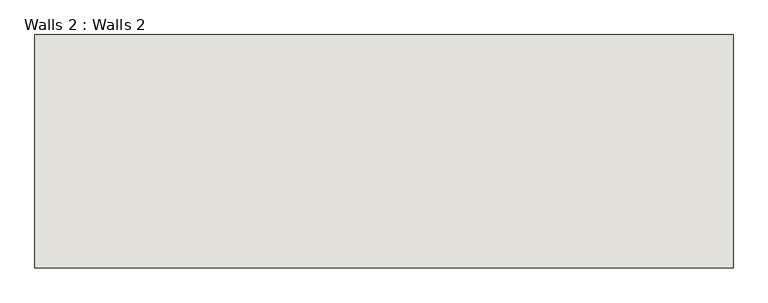
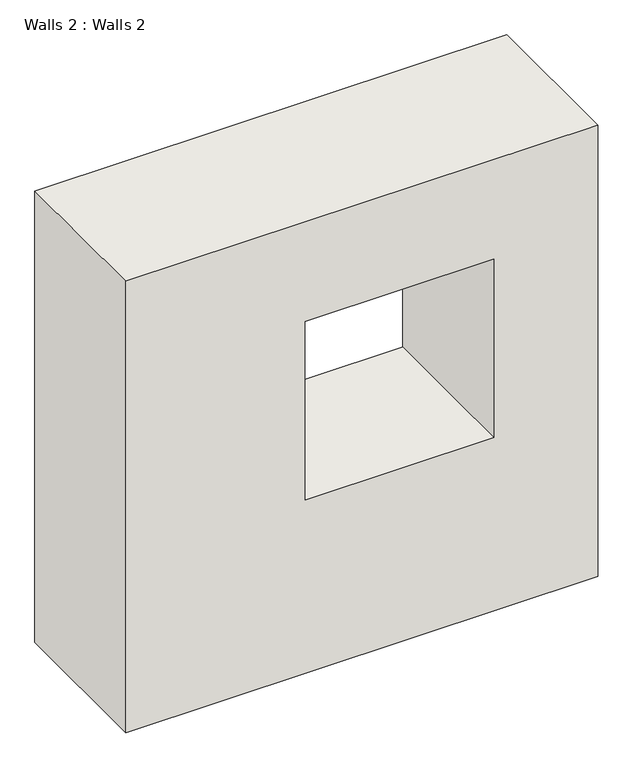
"""IFC4 building model written with IfcOpenShell, lengths in millimetres: wall geometry, Walls 2 : Walls 2."""

from ifc_helpers import new_model, si_unit, frame, origin, place, context, project, spatial, polyline, outline, extrude, source, transform, mapped, element, save


def walls_2_walls_2_253db866(model_context):
    return source(origin(), model_context, "Body", "SweptSolid", [
        extrude(outline(polyline([(3860.8, -8998.6105967), (3860.8, -12813.1931367), (0.0, -12813.1931367), (0.0, -8998.6105967), (3860.8, -8998.6105967)]), holes=[polyline([(1484.4102642, -11362.5013745), (3008.4102642, -11362.5013745), (3008.4102642, -9838.5013745), (1484.4102642, -9838.5013745), (1484.4102642, -11362.5013745)])]), frame((0.0, 1282.1739897, 0.0), z_axis=(0.0, 1.0, 0.0), x_axis=(0.0, 0.0, 1.0)), (0.0, 0.0, 1.0), 1274.1057169),
    ])


if __name__ == "__main__":
    model = new_model("IFC4")
    model_context = context("Model", 3, world=origin())
    ifc_project = project(units=[si_unit("LENGTHUNIT", "METRE", prefix="MILLI")], contexts=[model_context])
    site = spatial("IfcSite", under=ifc_project)
    building = spatial("IfcBuilding", under=site)
    placement = place(None, origin())
    walls_2_walls_2_shape = walls_2_walls_2_253db866(model_context)
    element("IfcWall", 1, ObjectType="Walls 2 : Walls 2", at=placement, inside=building, context=model_context, shape_type="MappedRepresentation", body=[
        mapped(walls_2_walls_2_shape, transform((0.0, 0.0, 0.0), x_axis=(1.0, 0.0, 0.0), y_axis=(0.0, 1.0, 0.0), z_axis=(0.0, 0.0, 1.0))),
    ])
    save(model, "model.ifc")

# Revit data of these elements
# Element 1 (IfcWall, "Walls 2 : Walls 2")
#   Materials on its faces: "Default Wall"
# Materials
#   "Default Wall": colour RGB 128 128 128, transparency 0
